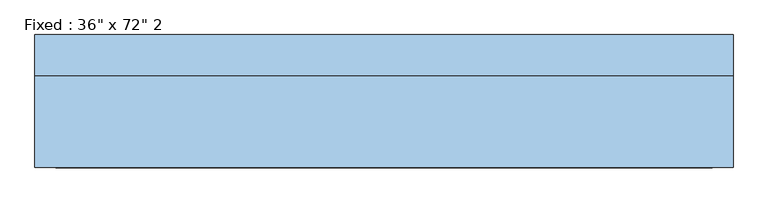
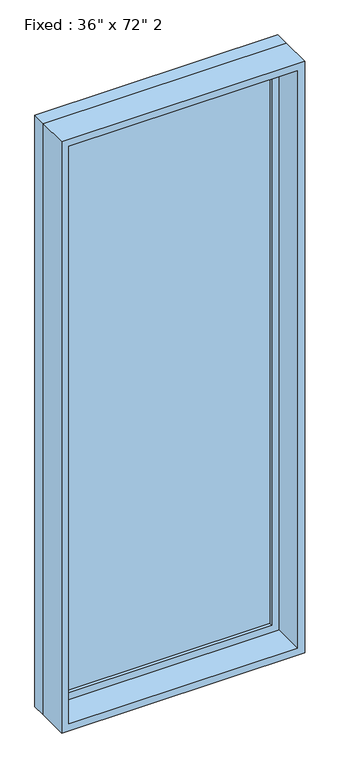
"""IFC4 building model written with IfcOpenShell, lengths in millimetres: window geometry."""

from ifc_helpers import new_model, si_unit, frame, origin, place, context, project, spatial, polyline, outline, extrude, source, transform, mapped, element, save


def window_1a213a25(model_context):
    return source(origin(), model_context, "Body", "SweptSolid", [
        extrude(outline(polyline([(431.8, 53.975), (-508.0, 53.975), (-508.0, 66.675), (431.8, 66.675), (431.8, 53.975)])), frame((0.0, 0.0, 368.3), z_axis=(0.0, 0.0, 1.0), x_axis=(1.0, 0.0, 0.0)), (0.0, 0.0, 1.0), 2616.2),
        extrude(outline(polyline([(3028.95, -552.45), (323.85, -552.45), (323.85, 476.25), (3028.95, 476.25), (3028.95, -552.45)]), holes=[polyline([(2984.5, -508.0), (2984.5, 431.8), (368.3, 431.8), (368.3, -508.0), (2984.5, -508.0)])]), frame((0.0, 38.1, 0.0), z_axis=(0.0, 1.0, 0.0), x_axis=(0.0, 0.0, 1.0)), (0.0, 0.0, 1.0), 44.45),
        extrude(outline(polyline([(3048.0, -571.5), (304.8, -571.5), (304.8, 495.3), (3048.0, 495.3), (3048.0, -571.5)]), holes=[polyline([(3016.25, -539.75), (3016.25, 463.55), (336.55, 463.55), (336.55, -539.75), (3016.25, -539.75)])]), frame((0.0, -101.6, 0.0), z_axis=(0.0, 1.0, 0.0), x_axis=(0.0, 0.0, 1.0)), (0.0, 0.0, 1.0), 139.7),
        extrude(outline(polyline([(3048.0, 495.3), (3048.0, -571.5), (304.8, -571.5), (304.8, 495.3), (3048.0, 495.3)]), holes=[polyline([(3028.95, 476.25), (323.85, 476.25), (323.85, -552.45), (3028.95, -552.45), (3028.95, 476.25)])]), frame((0.0, 38.1, 0.0), z_axis=(0.0, 1.0, 0.0), x_axis=(0.0, 0.0, 1.0)), (0.0, 0.0, 1.0), 63.5),
    ])


if __name__ == "__main__":
    model = new_model("IFC4")
    model_context = context("Model", 3, world=origin())
    ifc_project = project(units=[si_unit("LENGTHUNIT", "METRE", prefix="MILLI")], contexts=[model_context])
    site = spatial("IfcSite", under=ifc_project)
    building = spatial("IfcBuilding", under=site)
    placement = place(None, origin())
    window_shape = window_1a213a25(model_context)
    element("IfcWindow", 1, ObjectType="Fixed : 36\" x 72\" 2", at=placement, inside=building, context=model_context, shape_type="MappedRepresentation", body=[
        mapped(window_shape, transform((0.0, 0.0, 0.0), x_axis=(1.0, 0.0, 0.0), y_axis=(0.0, 1.0, 0.0), z_axis=(0.0, 0.0, 1.0))),
    ])
    save(model, "model.ifc")

# Revit data of these elements
# Type "Fixed : 36\" x 72\" 2"
#   Type Mark = "29"
#   Construction Type Id = "GSP4R"
#   Assembly Code = "B2020100"
#   Analytic Construction = "1/8 in Pilkington single glazing"
#   Visual Light Transmittance = 0.9
#   Solar Heat Gain Coefficient = 0.78
#   Heat Transfer Coefficient (U) = 3.6886 W/(m²·K)
#   Height = 9' - 0"
#   Default Sill Height = 1' - 0"
#   Width = 3' - 6"
#   Window Inset = 0' - 0 3/4"
#   Glass Pane Material = Glass
#   Sash Material = Iron, Ductile
#   Wall Closure = (empty or 0)
# Element 1 (IfcWindow, "Fixed : 36\" x 72\" 2")
#   Materials on its faces: "Iron, Ductile", "Glass"
# Materials
#   "Glass": class "Glass", colour RGB 0 128 192, transparency 0.75, Description = "Soda Lime Glass", Cost = 0
#   "Iron, Ductile": class "Metal", colour RGB 0 0 0, transparency 0, Description = "Ductile cast iron", Cost = 0
